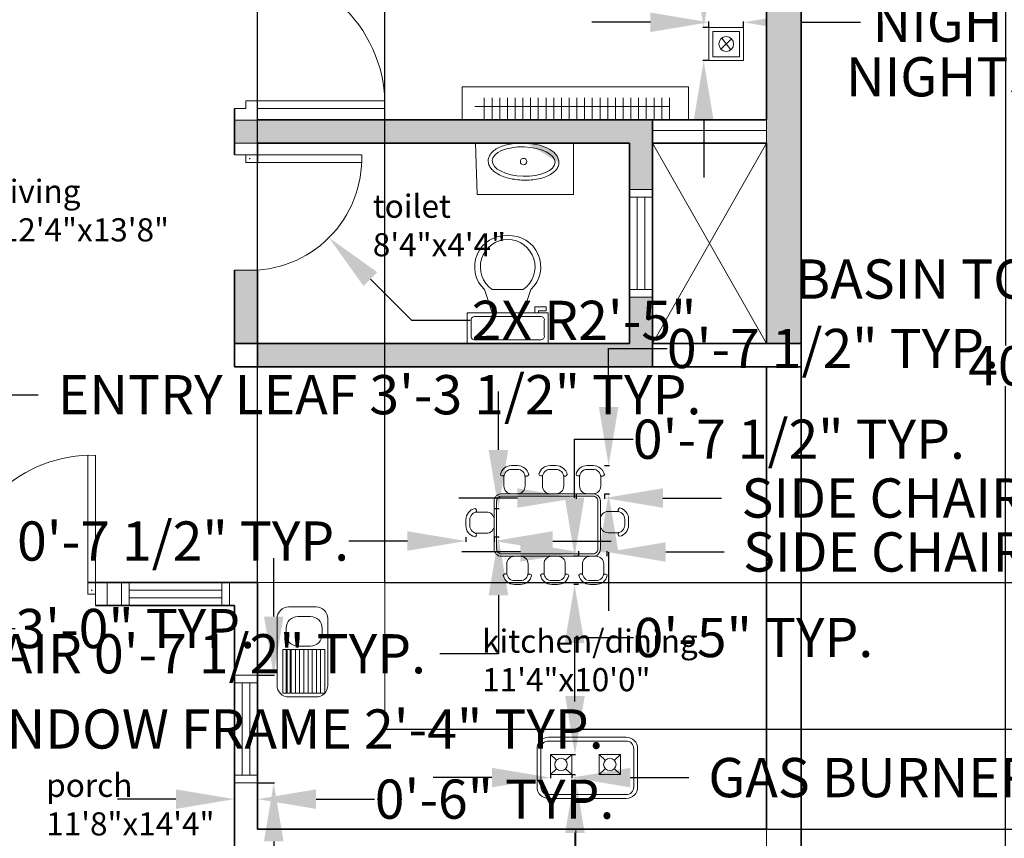
# Model space of a CAD drawing. Units: inches. Extents: x 19 to 15718, y 7 to 930.
# Tile 4 of 11: x 14988 to 15243, y 468 to 680. Entities that reach past the tile are written whole.
import ezdxf

# ---------------------------------------------------------------- set-up
doc = ezdxf.new("R2010")
doc.units = ezdxf.units.IN
doc.header["$MEASUREMENT"] = 0
for name, color, linetype, lineweight in [('A-ANNO-DIMS', 2, 'Continuous', 18), ('A-AREA-IDEN', 7, 'Continuous', 18), ('A-DOOR', 4, 'Continuous', 20), ('A-EQPM', 9, 'Continuous', 18), ('A-FLOR-CASE', 8, 'Continuous', 18), ('A-FLOR-FIXT', 9, 'Continuous', 18), ('A-FLOR-OPEN', 8, 'Continuous', 13), ('A-FURN', 8, 'Continuous', 18), ('A-GLAZ', 4, 'Continuous', 18), ('A-WALL', 7, 'Continuous', 35)]:
    doc.layers.add(name, color=color, linetype=linetype, lineweight=lineweight)
doc.layers.add('A-WALL-PATT', color=18, linetype='Continuous', lineweight=13, true_color=0x000000)
doc.styles.add('Annotative', font='arial.ttf')
doc.styles.get("Standard").update_dxf_attribs({"font": 'arial.ttf'})
doc.dimstyles.get("Standard").update_dxf_attribs({"dimtxt": 10.18, "dimasz": 15.18, "dimexe": 0.18, "dimexo": 0.0625, "dimgap": 0.09, "dimtad": 0, "dimtih": 1, "dimtoh": 1, "dimdec": 0, "dimzin": 0, "dimdsep": 46, "dimlunit": 3, "dimtxsty": 'Standard', "dimcen": 0.09, "dimadec": 0, "dimazin": 0, "dimtfac": 1, "dimtdec": 0, "dimtofl": 0, "dimtmove": 0, "dimatfit": 3, "dimfxl": 1, "dimtolj": 1, "dimtzin": 0, "dimarcsym": 0})

# ---------------------------------------------------------------- blocks, each defined once
blk = doc.blocks.new('*U2')
for p, q in [((9.5, -6), (9.5, -2)), ((-10, -8.5), (-8, -8.5)), ((-10, -9.5), (-10, -8.5)), ((-7, -9.5), (-10, -9.5)), ((-8, -8.5), (-8, -8)), ((-7, -8), (-7, -9.5)), ((-4, -8), (-6, -14)), ((4, -8), (6, -14)), ((4, -14), (-4, -14))]:
    blk.add_line(p, q)
blk.add_lwpolyline([(10.5, -8), (10.5, 0), (-10.5, 0), (-10.5, -8)], close=True)
for points in [[(-9.5, -2), (-9.5, -6)], [(8.5, -1), (-8.5, -1)], [(-8.5, -7), (8.5, -7)]]:
    blk.add_lwpolyline(points)
for centre, radius, start, end in [((-8.625, -1.875), 0.8839, 81.8699, 188.1301), ((8.625, -1.875), 0.8839, 351.8699, 98.1301), ((-8.625, -6.125), 0.8839, 171.869898, 278.1301), ((8.625, -6.125), 0.8839, 261.8699, 8.1301), ((-0.4772, -19.9188), 8.0953, 133.01722, 273.38), ((0.0374, -19.8731), 7.127, 124.50543, 269.7), ((-0.0373, -19.8731), 7.127, 270.3, 55.4946), ((0.4773, -19.9188), 8.0953, 266.62, 46.9828)]:
    blk.add_arc(centre, radius, start, end)
blk = doc.blocks.new('*D17')
at = {"layer": 'A-ANNO-DIMS', "color": 0, "lineweight": -2, "transparency": 16777216}
for p, q in [((15266.62, 830.27), (15243.58, 830.27)), ((15243.76, 815.09), (15243.76, 595.52)), ((15243.76, 365.38), (15243.76, 584.95)), ((15266.62, 350.2), (15243.58, 350.2))]:
    blk.add_line(p, q, dxfattribs=at)
at = {"layer": 'A-ANNO-DIMS', "color": 0, "transparency": 16777216}
for points in [[(15241.23, 815.09), (15246.29, 815.09), (15243.76, 830.27)], [(15241.23, 365.38), (15246.29, 365.38), (15243.76, 350.2)]]:
    blk.add_solid(points, dxfattribs=at)
at = {"layer": 'Defpoints', "color": 0, "transparency": 16777216}
for p in [(15266.68, 830.27), (15243.76, 350.2), (15266.68, 350.2)]:
    blk.add_point(p, dxfattribs=at)
at = {"layer": 'A-ANNO-DIMS', "color": 0, "transparency": 16777216, "insert": (15243.76, 590.24), "char_height": 10.18, "attachment_point": 5}
blk.add_mtext("\\A1;40'", dxfattribs=at)
blk = doc.blocks.new('DOOR-SWING-36IN')
for p, q in [((34.01, 3), (34.01, 39)), ((36.01, 6), (36.01, 39)), ((0.01, 6), (0.01, 0)), ((34.01, 6), (39.01, 6)), ((39.01, 6), (39.01, 0)), ((34.01, 3), (36.01, 3)), ((36.01, 3), (36.01, 0))]:
    blk.add_line(p, q)
blk.add_arc((35.01, 4), 35.01, 88.3634, 181.6366)
blk = doc.blocks.new('WIN-24IN-FRAME6')
for p, q in [((0, 28), (6, 28)), ((0, 26), (6, 26)), ((2, 26), (2, 2)), ((4, 26), (4, 2)), ((0, 2), (6, 2)), ((0, 0), (6, 0))]:
    blk.add_line(p, q)
blk = doc.blocks.new('CHAIR-DINING-LONG-SIDE-A')
blk.add_lwpolyline([(0, 5.06, -0.34468), (2.91, 7.33), (4.42, 7.33, -0.353049), (7.35, 4.97, -0.353049)], format="xyb")
blk.add_lwpolyline([(0.91, 4.33, -0.414214), (2.91, 6.33), (4.42, 6.33, -0.414214), (6.42, 4.33), (6.42, 2, -0.414214), (4.42, 0), (2.91, 0, -0.414214), (0.91, 2)], format="xyb", close=True)
for centre, radius, start, end in [((0.54, 5.15), 0.548, 190.2724, 321.8719), ((6.8, 5.16), 0.588, 223.9333, 340.5026)]:
    blk.add_arc(centre, radius, start, end)
blk = doc.blocks.new('CHAIR-DINING-LONG-SIDE-B')
blk.add_lwpolyline([(6.44, 3, -0.414214), (4.44, 1), (2.93, 1, -0.414214), (0.93, 3), (0.93, 5.33, -0.414214), (2.93, 7.33), (4.44, 7.33, -0.414214), (6.44, 5.33)], format="xyb", close=True)
blk.add_lwpolyline([(7.35, 2.28, -0.34468), (4.44, 0), (2.93, 0, -0.353049), (0, 2.37, -0.353049)], format="xyb")
for centre, radius, start, end in [((0.55, 2.17), 0.588, 43.9333, 160.5026), ((6.81, 2.18), 0.548, 10.2724, 141.8719)]:
    blk.add_arc(centre, radius, start, end)
blk = doc.blocks.new('CHAIR-DINING-END')
blk.add_lwpolyline([(4.33, 6.44, -0.414214), (6.33, 4.44), (6.33, 2.93, -0.414214), (4.33, 0.93), (2, 0.93, -0.414214), (0, 2.93), (0, 4.44, -0.414214), (2, 6.44)], format="xyb", close=True)
blk.add_lwpolyline([(5.06, 7.35, -0.34468), (7.33, 4.44), (7.33, 2.93, -0.353049), (4.97, 0, -0.353049)], format="xyb")
for centre, radius, start, end in [((5.15, 6.81), 0.548, 100.2724, 231.8719), ((5.16, 0.55), 0.588, 133.9333, 250.5026)]:
    blk.add_arc(centre, radius, start, end)
blk = doc.blocks.new('NIGHTSTAND-SQUARE')
for p, q in [((5.89, 5.61), (3.09, 2.97)), ((3.32, 5.82), (5.66, 2.76)), ((3.09, 2.97), (3.09, 2.97))]:
    blk.add_line(p, q)
for points in [[(0, 8.58), (8.98, 8.58), (8.98, 0), (0, 0)], [(1, 7.58), (7.98, 7.58), (7.98, 1), (1, 1)]]:
    blk.add_lwpolyline(points, close=True)
blk.add_circle((4.49, 4.29), 1.92)
blk = doc.blocks.new('HOB-GAS-BURNER')
for p, q in [((0, 5.15), (1.58, 3.68)), ((3.94, 3.69), (5.54, 5.15)), ((1.58, 3.68), (1.58, 3.68)), ((0, 0), (1.58, 1.47)), ((5.54, 0), (3.95, 1.47))]:
    blk.add_line(p, q)
blk.add_lwpolyline([(0, 5.15), (0, 5.15), (5.54, 5.15), (5.54, 5.15), (5.54, 0), (5.54, 0), (0, 0), (0, 0)], close=True)
blk.add_circle((2.77, 2.57), 1.62)
blk = doc.blocks.new('*D36')
at = {"layer": 'A-ANNO-DIMS', "color": 0, "lineweight": -2, "transparency": 16777216}
for p, q in [((15054.04, 525.18), (15054.04, 540.36)), ((15049.9, 510), (15054.22, 510)), ((15049.9, 482), (15054.22, 482)), ((15054.04, 466.82), (15054.04, 451.64))]:
    blk.add_line(p, q, dxfattribs=at)
at = {"layer": 'A-ANNO-DIMS', "color": 0, "transparency": 16777216}
for points in [[(15051.51, 525.18), (15056.57, 525.18), (15054.04, 510)], [(15051.51, 466.82), (15056.57, 466.82), (15054.04, 482)]]:
    blk.add_solid(points, dxfattribs=at)
at = {"layer": 'Defpoints', "color": 0, "transparency": 16777216}
for p in [(15049.84, 510), (15054.04, 510), (15049.84, 482)]:
    blk.add_point(p, dxfattribs=at)
at = {"layer": 'A-ANNO-DIMS', "color": 0, "transparency": 16777216, "insert": (15054.04, 496), "char_height": 10.18, "attachment_point": 5}
blk.add_mtext('\\A1;WINDOW FRAME 2\'-4" TYP.', dxfattribs=at)
blk = doc.blocks.new('*D37')
at = {"layer": 'A-ANNO-DIMS', "color": 0, "lineweight": -2, "transparency": 16777216}
for p, q in [((15043.84, 481.93), (15043.84, 477.62)), ((15049.84, 481.93), (15049.84, 477.62)), ((15028.66, 477.8), (15013.48, 477.8)), ((15065.02, 477.8), (15080.2, 477.8))]:
    blk.add_line(p, q, dxfattribs=at)
at = {"layer": 'A-ANNO-DIMS', "color": 0, "transparency": 16777216}
for points in [[(15028.66, 480.33), (15028.66, 475.27), (15043.84, 477.8)], [(15065.02, 480.33), (15065.02, 475.27), (15049.84, 477.8)]]:
    blk.add_solid(points, dxfattribs=at)
at = {"layer": 'Defpoints', "color": 0, "transparency": 16777216}
for p in [(15043.84, 482), (15049.84, 482), (15049.84, 477.8)]:
    blk.add_point(p, dxfattribs=at)
at = {"layer": 'A-ANNO-DIMS', "color": 0, "transparency": 16777216, "insert": (15111.31, 477.8), "char_height": 10.18, "attachment_point": 5}
blk.add_mtext('\\A1;0\'-6" TYP.', dxfattribs=at)
blk = doc.blocks.new('*D40')
at = {"layer": 'A-ANNO-DIMS', "color": 0, "lineweight": -2, "transparency": 16777216}
for p, q in [((15132.43, 556.96), (15132.43, 555.74)), ((15139.78, 556.96), (15139.78, 555.74)), ((15117.25, 555.92), (15102.07, 555.92)), ((15154.96, 555.92), (15170.14, 555.92))]:
    blk.add_line(p, q, dxfattribs=at)
at = {"layer": 'A-ANNO-DIMS', "color": 0, "transparency": 16777216}
for points in [[(15117.25, 558.45), (15117.25, 553.39), (15132.43, 555.92)], [(15154.96, 558.45), (15154.96, 553.39), (15139.78, 555.92)]]:
    blk.add_solid(points, dxfattribs=at)
at = {"layer": 'Defpoints', "color": 0, "transparency": 16777216}
for p in [(15132.43, 557.02), (15139.78, 557.02), (15139.78, 555.92)]:
    blk.add_point(p, dxfattribs=at)
at = {"layer": 'A-ANNO-DIMS', "color": 0, "transparency": 16777216, "insert": (15262.49, 555.92), "char_height": 10.18, "attachment_point": 5}
blk.add_mtext('\\A1;SIDE CHAIR A 0\'-7 1/2" TYP.', dxfattribs=at)
blk = doc.blocks.new('*D41')
at = {"layer": 'A-ANNO-DIMS', "color": 0, "lineweight": -2, "transparency": 16777216}
for p, q in [((15140.89, 579.54), (15140.89, 594.72)), ((15140.89, 594.72), (15156.07, 594.72)), ((15139.85, 564.36), (15141.07, 564.36)), ((15139.85, 557.02), (15141.07, 557.02)), ((15140.89, 541.84), (15140.89, 526.66))]:
    blk.add_line(p, q, dxfattribs=at)
at = {"layer": 'A-ANNO-DIMS', "color": 0, "transparency": 16777216}
for points in [[(15138.36, 579.54), (15143.42, 579.54), (15140.89, 564.36)], [(15138.36, 541.84), (15143.42, 541.84), (15140.89, 557.02)]]:
    blk.add_solid(points, dxfattribs=at)
at = {"layer": 'Defpoints', "color": 0, "transparency": 16777216}
for p in [(15139.78, 564.36), (15140.89, 564.36), (15139.78, 557.02)]:
    blk.add_point(p, dxfattribs=at)
at = {"layer": 'A-ANNO-DIMS', "color": 0, "transparency": 16777216, "insert": (15199.04, 594.72), "char_height": 10.18, "attachment_point": 5}
blk.add_mtext('\\A1;0\'-7 1/2" TYP.', dxfattribs=at)
blk = doc.blocks.new('*D42')
at = {"layer": 'A-ANNO-DIMS', "color": 0, "lineweight": -2, "transparency": 16777216}
for p, q in [((15117.99, 541.92), (15102.81, 541.92)), ((15133.17, 540.88), (15133.17, 542.1)), ((15140.52, 540.88), (15140.52, 542.1)), ((15155.7, 541.92), (15170.88, 541.92))]:
    blk.add_line(p, q, dxfattribs=at)
at = {"layer": 'A-ANNO-DIMS', "color": 0, "transparency": 16777216}
for points in [[(15117.99, 544.45), (15117.99, 539.39), (15133.17, 541.92)], [(15155.7, 544.45), (15155.7, 539.39), (15140.52, 541.92)]]:
    blk.add_solid(points, dxfattribs=at)
at = {"layer": 'Defpoints', "color": 0, "transparency": 16777216}
for p in [(15140.52, 541.92), (15133.17, 540.82), (15140.52, 540.82)]:
    blk.add_point(p, dxfattribs=at)
at = {"layer": 'A-ANNO-DIMS', "color": 0, "transparency": 16777216, "insert": (15263.22, 541.92), "char_height": 10.18, "attachment_point": 5}
blk.add_mtext('\\A1;SIDE CHAIR B 0\'-7 1/2" TYP.', dxfattribs=at)
blk = doc.blocks.new('*D43')
at = {"layer": 'A-ANNO-DIMS', "color": 0, "lineweight": -2, "transparency": 16777216}
for p, q in [((15132.06, 556), (15132.06, 571.18)), ((15132.06, 571.18), (15147.24, 571.18)), ((15133.1, 540.82), (15131.88, 540.82)), ((15133.1, 533.49), (15131.88, 533.49)), ((15132.06, 518.31), (15132.06, 503.13))]:
    blk.add_line(p, q, dxfattribs=at)
at = {"layer": 'A-ANNO-DIMS', "color": 0, "transparency": 16777216}
for points in [[(15129.53, 556), (15134.59, 556), (15132.06, 540.82)], [(15129.53, 518.31), (15134.59, 518.31), (15132.06, 533.49)]]:
    blk.add_solid(points, dxfattribs=at)
at = {"layer": 'Defpoints', "color": 0, "transparency": 16777216}
for p in [(15132.06, 540.82), (15133.17, 540.82), (15133.17, 533.49)]:
    blk.add_point(p, dxfattribs=at)
at = {"layer": 'A-ANNO-DIMS', "color": 0, "transparency": 16777216, "insert": (15190.22, 571.18), "char_height": 10.18, "attachment_point": 5}
blk.add_mtext('\\A1;0\'-7 1/2" TYP.', dxfattribs=at)
blk = doc.blocks.new('*D46')
at = {"layer": 'A-ANNO-DIMS', "color": 0, "lineweight": -2, "transparency": 16777216}
for p, q in [((15358.25, 608.29), (15358.25, 612.91)), ((15388.25, 608.29), (15388.25, 612.91)), ((15343.07, 612.73), (15327.89, 612.73)), ((15403.43, 612.73), (15418.61, 612.73))]:
    blk.add_line(p, q, dxfattribs=at)
at = {"layer": 'A-ANNO-DIMS', "color": 0, "transparency": 16777216}
for points in [[(15343.07, 615.26), (15343.07, 610.2), (15358.25, 612.73)], [(15403.43, 615.26), (15403.43, 610.2), (15388.25, 612.73)]]:
    blk.add_solid(points, dxfattribs=at)
at = {"layer": 'Defpoints', "color": 0, "transparency": 16777216}
for p in [(15358.25, 612.73), (15358.25, 608.23), (15388.25, 608.23)]:
    blk.add_point(p, dxfattribs=at)
at = {"layer": 'A-ANNO-DIMS', "color": 0, "transparency": 16777216, "insert": (15257.09, 612.73), "char_height": 10.18, "attachment_point": 5}
blk.add_mtext('\\A1;BASIN TOP 2\'-6" TYP.', dxfattribs=at)
blk = doc.blocks.new('*D50')
at = {"layer": 'A-ANNO-DIMS', "color": 0, "lineweight": -2, "transparency": 16777216}
for p, q in [((14977.77, 567.55), (14977.77, 582.73)), ((14977.77, 582.73), (14992.95, 582.73)), ((14971.9, 567.55), (14977.95, 567.55)), ((14977.77, 543.18), (14977.77, 552.37)), ((14971.9, 528), (14977.95, 528))]:
    blk.add_line(p, q, dxfattribs=at)
at = {"layer": 'A-ANNO-DIMS', "color": 0, "transparency": 16777216}
for points in [[(14975.24, 552.37), (14980.3, 552.37), (14977.77, 567.55)], [(14975.24, 543.18), (14980.3, 543.18), (14977.77, 528)]]:
    blk.add_solid(points, dxfattribs=at)
at = {"layer": 'Defpoints', "color": 0, "transparency": 16777216}
for p in [(14971.84, 567.55), (14977.77, 567.55), (14971.84, 528)]:
    blk.add_point(p, dxfattribs=at)
at = {"layer": 'A-ANNO-DIMS', "color": 0, "transparency": 16777216, "insert": (15081.49, 582.73), "char_height": 10.18, "attachment_point": 5}
blk.add_mtext('\\A1;ENTRY LEAF 3\'-3 1/2" TYP.', dxfattribs=at)
blk = doc.blocks.new('*D51')
at = {"layer": 'A-ANNO-DIMS', "color": 0, "lineweight": -2, "transparency": 16777216}
for p, q in [((14935.84, 527.93), (14935.84, 521.88)), ((14971.84, 527.93), (14971.84, 521.88)), ((14951.02, 522.06), (14956.66, 522.06)), ((14971.84, 522.06), (14987.02, 522.06))]:
    blk.add_line(p, q, dxfattribs=at)
at = {"layer": 'A-ANNO-DIMS', "color": 0, "transparency": 16777216}
for points in [[(14951.02, 524.59), (14951.02, 519.53), (14935.84, 522.06)], [(14956.66, 524.59), (14956.66, 519.53), (14971.84, 522.06)]]:
    blk.add_solid(points, dxfattribs=at)
at = {"layer": 'Defpoints', "color": 0, "transparency": 16777216}
for p in [(14935.84, 528), (14971.84, 528), (14971.84, 522.06)]:
    blk.add_point(p, dxfattribs=at)
at = {"layer": 'A-ANNO-DIMS', "color": 0, "transparency": 16777216, "insert": (15018.13, 522.06), "char_height": 10.18, "attachment_point": 5}
blk.add_mtext('\\A1;3\'-0" TYP.', dxfattribs=at)
blk = doc.blocks.new('*D54')
at = {"layer": 'A-ANNO-DIMS', "color": 0, "lineweight": -2, "transparency": 16777216}
for p, q in [((15112.3, 568.4), (15112.3, 583.58)), ((15111.26, 553.22), (15112.48, 553.22)), ((15111.26, 545.87), (15112.48, 545.87)), ((15112.3, 530.69), (15112.3, 515.51)), ((15112.3, 515.51), (15097.12, 515.51))]:
    blk.add_line(p, q, dxfattribs=at)
at = {"layer": 'A-ANNO-DIMS', "color": 0, "transparency": 16777216}
for points in [[(15109.77, 568.4), (15114.83, 568.4), (15112.3, 553.22)], [(15109.77, 530.69), (15114.83, 530.69), (15112.3, 545.87)]]:
    blk.add_solid(points, dxfattribs=at)
at = {"layer": 'Defpoints', "color": 0, "transparency": 16777216}
for p in [(15111.2, 553.22), (15111.2, 545.87), (15112.3, 545.87)]:
    blk.add_point(p, dxfattribs=at)
at = {"layer": 'A-ANNO-DIMS', "color": 0, "transparency": 16777216, "insert": (15013.32, 515.51), "char_height": 10.18, "attachment_point": 5}
blk.add_mtext('\\A1;END CHAIR 0\'-7 1/2" TYP.', dxfattribs=at)
blk = doc.blocks.new('*D55')
at = {"layer": 'A-ANNO-DIMS', "color": 0, "lineweight": -2, "transparency": 16777216}
for p, q in [((15088.69, 544.76), (15073.51, 544.76)), ((15103.87, 545.8), (15103.87, 544.58)), ((15111.2, 545.8), (15111.2, 544.58)), ((15126.38, 544.76), (15141.56, 544.76))]:
    blk.add_line(p, q, dxfattribs=at)
at = {"layer": 'A-ANNO-DIMS', "color": 0, "transparency": 16777216}
for points in [[(15088.69, 547.29), (15088.69, 542.23), (15103.87, 544.76)], [(15126.38, 547.29), (15126.38, 542.23), (15111.2, 544.76)]]:
    blk.add_solid(points, dxfattribs=at)
at = {"layer": 'Defpoints', "color": 0, "transparency": 16777216}
for p in [(15103.87, 545.87), (15103.87, 544.76), (15111.2, 545.87)]:
    blk.add_point(p, dxfattribs=at)
at = {"layer": 'A-ANNO-DIMS', "color": 0, "transparency": 16777216, "insert": (15030.53, 544.76), "char_height": 10.18, "attachment_point": 5}
blk.add_mtext('\\A1;0\'-7 1/2" TYP.', dxfattribs=at)
blk = doc.blocks.new('*D56')
at = {"layer": 'A-ANNO-DIMS', "color": 0, "lineweight": -2, "transparency": 16777216}
for p, q in [((15151.7, 679.35), (15136.52, 679.35)), ((15166.88, 678.06), (15166.88, 679.53)), ((15175.86, 678.06), (15175.86, 679.53)), ((15191.04, 679.35), (15206.22, 679.35))]:
    blk.add_line(p, q, dxfattribs=at)
at = {"layer": 'A-ANNO-DIMS', "color": 0, "transparency": 16777216}
for points in [[(15151.7, 681.88), (15151.7, 676.82), (15166.88, 679.35)], [(15191.04, 681.88), (15191.04, 676.82), (15175.86, 679.35)]]:
    blk.add_solid(points, dxfattribs=at)
at = {"layer": 'Defpoints', "color": 0, "transparency": 16777216}
for p in [(15175.86, 679.35), (15166.88, 678), (15175.86, 678)]:
    blk.add_point(p, dxfattribs=at)
at = {"layer": 'A-ANNO-DIMS', "color": 0, "transparency": 16777216, "insert": (15285.29, 679.35), "char_height": 10.18, "attachment_point": 5}
blk.add_mtext('\\A1;NIGHTSTAND 0\'-9" TYP.', dxfattribs=at)
blk = doc.blocks.new('*D57')
at = {"layer": 'A-ANNO-DIMS', "color": 0, "lineweight": -2, "transparency": 16777216}
for p, q in [((15165.53, 693.18), (15165.53, 708.36)), ((15165.53, 708.36), (15180.71, 708.36)), ((15166.82, 678), (15165.35, 678)), ((15166.82, 669.42), (15165.35, 669.42)), ((15165.53, 654.24), (15165.53, 639.06))]:
    blk.add_line(p, q, dxfattribs=at)
at = {"layer": 'A-ANNO-DIMS', "color": 0, "transparency": 16777216}
for points in [[(15163, 693.18), (15168.06, 693.18), (15165.53, 678)], [(15163, 654.24), (15168.06, 654.24), (15165.53, 669.42)]]:
    blk.add_solid(points, dxfattribs=at)
at = {"layer": 'Defpoints', "color": 0, "transparency": 16777216}
for p in [(15165.53, 678), (15166.88, 678), (15166.88, 669.42)]:
    blk.add_point(p, dxfattribs=at)
at = {"layer": 'A-ANNO-DIMS', "color": 0, "transparency": 16777216, "insert": (15223.69, 708.36), "char_height": 10.18, "attachment_point": 5}
blk.add_mtext('\\A1;0\'-8 1/2" TYP.', dxfattribs=at)
blk = doc.blocks.new('*D58')
at = {"layer": 'A-ANNO-DIMS', "color": 0, "lineweight": -2, "transparency": 16777216}
for p, q in [((15278.41, 688.79), (15278.41, 703.97)), ((15280.87, 673.61), (15278.23, 673.61)), ((15280.87, 656.82), (15278.23, 656.82)), ((15278.41, 641.64), (15278.41, 626.46))]:
    blk.add_line(p, q, dxfattribs=at)
at = {"layer": 'A-ANNO-DIMS', "color": 0, "transparency": 16777216}
for points in [[(15275.88, 688.79), (15280.94, 688.79), (15278.41, 673.61)], [(15275.88, 641.64), (15280.94, 641.64), (15278.41, 656.82)]]:
    blk.add_solid(points, dxfattribs=at)
at = {"layer": 'Defpoints', "color": 0, "transparency": 16777216}
for p in [(15278.41, 673.61), (15280.93, 673.61), (15280.93, 656.82)]:
    blk.add_point(p, dxfattribs=at)
at = {"layer": 'A-ANNO-DIMS', "color": 0, "transparency": 16777216, "insert": (15278.41, 665.21), "char_height": 10.18, "attachment_point": 5}
blk.add_mtext('\\A1;NIGHTSTAND 1\'-5" TYP.', dxfattribs=at)
blk = doc.blocks.new('*D60')
at = {"layer": 'A-ANNO-DIMS', "color": 0, "lineweight": -2, "transparency": 16777216}
for p, q in [((15110.6, 483.39), (15095.42, 483.39)), ((15125.78, 484.16), (15125.78, 483.21)), ((15131.32, 484.16), (15131.32, 483.21)), ((15146.5, 483.39), (15161.68, 483.39))]:
    blk.add_line(p, q, dxfattribs=at)
at = {"layer": 'A-ANNO-DIMS', "color": 0, "transparency": 16777216}
for points in [[(15110.6, 485.92), (15110.6, 480.86), (15125.78, 483.39)], [(15146.5, 485.92), (15146.5, 480.86), (15131.32, 483.39)]]:
    blk.add_solid(points, dxfattribs=at)
at = {"layer": 'Defpoints', "color": 0, "transparency": 16777216}
for p in [(15125.78, 484.23), (15131.32, 484.23), (15131.32, 483.39)]:
    blk.add_point(p, dxfattribs=at)
at = {"layer": 'A-ANNO-DIMS', "color": 0, "transparency": 16777216, "insert": (15253.56, 483.39), "char_height": 10.18, "attachment_point": 5}
blk.add_mtext('\\A1;GAS BURNER 0\'-5 1/2" TYP.', dxfattribs=at)
blk = doc.blocks.new('*D61')
at = {"layer": 'A-ANNO-DIMS', "color": 0, "lineweight": -2, "transparency": 16777216}
for p, q in [((15132.15, 504.55), (15132.15, 519.73)), ((15132.15, 519.73), (15147.33, 519.73)), ((15131.38, 489.37), (15132.33, 489.37)), ((15131.38, 484.23), (15132.33, 484.23)), ((15132.15, 469.05), (15132.15, 453.87))]:
    blk.add_line(p, q, dxfattribs=at)
at = {"layer": 'A-ANNO-DIMS', "color": 0, "transparency": 16777216}
for points in [[(15129.62, 504.55), (15134.68, 504.55), (15132.15, 489.37)], [(15129.62, 469.05), (15134.68, 469.05), (15132.15, 484.23)]]:
    blk.add_solid(points, dxfattribs=at)
at = {"layer": 'Defpoints', "color": 0, "transparency": 16777216}
for p in [(15131.32, 489.37), (15132.15, 489.37), (15131.32, 484.23)]:
    blk.add_point(p, dxfattribs=at)
at = {"layer": 'A-ANNO-DIMS', "color": 0, "transparency": 16777216, "insert": (15178.44, 519.73), "char_height": 10.18, "attachment_point": 5}
blk.add_mtext('\\A1;0\'-5" TYP.', dxfattribs=at)
blk = doc.blocks.new('*D78')
at = {"layer": 'A-ANNO-DIMS', "color": 0, "lineweight": -2, "transparency": 16777216}
for p, q in [((15049.84, 534.06), (15049.84, 923.53)), ((15065.02, 923.35), (15067.65, 923.35)), ((15082.83, 534.06), (15082.83, 923.53)), ((15082.83, 923.35), (15098.01, 923.35))]:
    blk.add_line(p, q, dxfattribs=at)
at = {"layer": 'A-ANNO-DIMS', "color": 0, "transparency": 16777216}
for points in [[(15065.02, 925.88), (15065.02, 920.82), (15049.84, 923.35)], [(15067.65, 925.88), (15067.65, 920.82), (15082.83, 923.35)]]:
    blk.add_solid(points, dxfattribs=at)
at = {"layer": 'Defpoints', "color": 0, "transparency": 16777216}
for p in [(15082.83, 923.35), (15049.84, 534), (15082.83, 534)]:
    blk.add_point(p, dxfattribs=at)
at = {"layer": 'A-ANNO-DIMS', "color": 0, "transparency": 16777216, "insert": (15111.72, 923.35), "char_height": 10.18, "attachment_point": 5}
blk.add_mtext('\\A1;2\'-9"', dxfattribs=at)
blk = doc.blocks.new('*D79')
at = {"layer": 'A-ANNO-DIMS', "color": 0, "lineweight": -2, "transparency": 16777216}
for p, q in [((15602.03, 534), (15602.03, 549.18)), ((15602.03, 549.18), (15617.21, 549.18)), ((15082.89, 534), (15602.21, 534)), ((15602.03, 511.14), (15602.03, 518.82)), ((15082.89, 495.96), (15602.21, 495.96))]:
    blk.add_line(p, q, dxfattribs=at)
at = {"layer": 'A-ANNO-DIMS', "color": 0, "transparency": 16777216}
for points in [[(15599.5, 518.82), (15604.56, 518.82), (15602.03, 534)], [(15599.5, 511.14), (15604.56, 511.14), (15602.03, 495.96)]]:
    blk.add_solid(points, dxfattribs=at)
at = {"layer": 'Defpoints', "color": 0, "transparency": 16777216}
for p in [(15082.83, 534), (15602.03, 534), (15082.83, 495.96)]:
    blk.add_point(p, dxfattribs=at)
at = {"layer": 'A-ANNO-DIMS', "color": 0, "transparency": 16777216, "insert": (15630.83, 549.18), "char_height": 10.18, "attachment_point": 5}
blk.add_mtext('\\A1;3\'-2"', dxfattribs=at)
blk = doc.blocks.new('*D80')
at = {"layer": 'A-ANNO-DIMS', "color": 0, "lineweight": -2, "transparency": 16777216}
for p, q in [((15602.030581, 511.142303), (15602.030581, 526.322303)), ((15181.899116, 495.962303), (15602.210581, 495.962303)), ((15181.899116, 469.995573), (15602.210581, 469.995573)), ((15602.030581, 454.815573), (15602.030581, 439.635573))]:
    blk.add_line(p, q, dxfattribs=at)
at = {"layer": 'A-ANNO-DIMS', "color": 0, "transparency": 16777216}
for points in [[(15599.500581, 511.142303), (15604.560581, 511.142303), (15602.030581, 495.962303)], [(15599.500581, 454.815573), (15604.560581, 454.815573), (15602.030581, 469.995573)]]:
    blk.add_solid(points, dxfattribs=at)
at = {"layer": 'Defpoints', "color": 0, "transparency": 16777216}
for p in [(15181.836616, 495.962303), (15602.030581, 495.962303), (15181.836616, 469.995573)]:
    blk.add_point(p, dxfattribs=at)
at = {"layer": 'A-ANNO-DIMS', "color": 0, "transparency": 16777216, "insert": (15602.030581, 482.978938), "char_height": 10.18, "attachment_point": 5}
blk.add_mtext('\\A1;2\'-2"', dxfattribs=at)
blk = doc.blocks.new('*D87')
at = {"layer": 'A-ANNO-DIMS', "color": 0, "lineweight": -2, "transparency": 16777216}
for p, q in [((14946.77, 579.52), (14961.95, 579.52)), ((14961.95, 579.52), (14972.37, 568.49)), ((15006.75, 532), (15006.93, 532)), ((15006.84, 531.91), (15006.84, 532.09))]:
    blk.add_line(p, q, dxfattribs=at)
at = {"layer": 'A-ANNO-DIMS', "color": 0, "transparency": 16777216}
blk.add_solid([(14974.21, 570.22), (14970.53, 566.75), (14982.79, 557.45)], dxfattribs=at)
at = {"layer": 'Defpoints', "color": 0, "transparency": 16777216}
for p in [(14982.79, 557.45), (15006.84, 532)]:
    blk.add_point(p, dxfattribs=at)
at = {"layer": 'A-ANNO-DIMS', "color": 0, "transparency": 16777216, "insert": (14913.39, 579.52), "char_height": 10.18, "attachment_point": 5}
blk.add_mtext('\\A1;5X R2\'-11"', dxfattribs=at)
blk = doc.blocks.new('*D88')
at = {"layer": 'A-ANNO-DIMS', "color": 0, "lineweight": -2, "transparency": 16777216}
for p, q in [((15047.75, 644), (15047.93, 644)), ((15047.84, 643.91), (15047.84, 644.09)), ((15089.82, 602.01), (15079.09, 612.74)), ((15105, 602.01), (15089.82, 602.01))]:
    blk.add_line(p, q, dxfattribs=at)
at = {"layer": 'A-ANNO-DIMS', "color": 0, "transparency": 16777216}
blk.add_solid([(15080.88, 614.53), (15077.3, 610.95), (15068.35, 623.48)], dxfattribs=at)
at = {"layer": 'Defpoints', "color": 0, "transparency": 16777216}
for p in [(15047.84, 644), (15068.35, 623.48)]:
    blk.add_point(p, dxfattribs=at)
at = {"layer": 'A-ANNO-DIMS', "color": 0, "transparency": 16777216, "insert": (15134.52, 602.01), "char_height": 10.18, "attachment_point": 5}
blk.add_mtext('\\A1;2X R2\'-5"', dxfattribs=at)

msp = doc.modelspace()

# ---------------------------------------------------------------- hatches: boundary and pattern name
at = {"layer": 'A-WALL-PATT'}
h = msp.add_hatch(color=256, dxfattribs=at)
h.dxf.hatch_style = 1
h.paths.add_polyline_path([(15190.84, 837), (14890.84, 837), (14890.84, 357), (14899.84, 357), (14899.84, 366), (14899.84, 528), (14904.84, 528), (14904.84, 534), (14899.84, 534), (14899.84, 698), (15004.84, 698), (15004.84, 701, -0.014283), (15004.84, 703), (15004.84, 704), (14899.84, 704), (14899.84, 828), (14987.26, 828), (15043.84, 828), (15049.84, 828), (15075.84, 828), (15081.84, 828), (15181.84, 828), (15181.84, 780), (15114.84, 780), (15114.84, 779, -0.017236), (15114.84, 777), (15114.84, 774), (15181.84, 774), (15181.84, 654), (15181.84, 648), (15181.84, 596), (15190.84, 596)])
h.paths.add_polyline_path([(15190.84, 590), (15181.84, 590), (15181.84, 470), (15181.84, 464), (15181.84, 361.43), (14991.9, 361.43), (14991.5, 357), (15190.84, 357)], flags=0)
h.paths.add_polyline_path([(15152.29, 608), (15146.29, 608), (15146.29, 596), (15049.84, 596), (15049.84, 590), (15152.29, 590)], flags=17)
h.paths.add_polyline_path([(15049.84, 615), (15048.84, 615, -0.017236), (15046.84, 615), (15043.84, 615), (15043.84, 596), (15049.84, 596)], flags=17)
edge = h.paths.add_edge_path(flags=17)
edge.add_line((15152.29, 654), (15049.84, 654))
edge.add_line((15049.84, 654), (15043.84, 654))
edge.add_line((15043.84, 654), (15043.84, 648))
edge.add_line((15043.84, 648), (15049.84, 648))
edge.add_line((15049.84, 648), (15075.84, 648))
edge.add_line((15075.84, 648), (15081.84, 648))
edge.add_line((15081.84, 648), (15117.26, 648))
edge.add_spline(control_points=[(15117.26, 648), (15117.59, 648.02), (15117.94, 648.03), (15118.71, 648.04), (15119.15, 648.02), (15119.59, 648)], knot_values=[1.499122, 1.499122, 1.499122, 1.499122, 1.618335, 1.618335, 1.770388, 1.770388, 1.770388, 1.770388], degree=3, periodic=0)
edge.add_spline(control_points=[(15127.99, 642.93), (15128, 643.28), (15127.95, 643.62), (15127.73, 644.26), (15127.57, 644.57), (15127.16, 645.13), (15126.92, 645.39), (15126.04, 646.16), (15125.28, 646.6), (15123.53, 647.31), (15122.55, 647.59), (15120.88, 647.88), (15120.24, 647.95), (15119.59, 648)], knot_values=[0, 0, 0, 0, 0.172075, 0.172075, 0.344149, 0.344149, 0.516224, 0.516224, 0.894541, 0.894541, 1.272858, 1.272858, 1.499122, 1.499122, 1.499122, 1.499122], degree=3, periodic=0)
edge.add_line((15119.59, 648), (15146.29, 648))
edge.add_line((15146.29, 648), (15146.29, 636))
edge.add_line((15146.29, 636), (15152.29, 636))
edge.add_line((15152.29, 636), (15152.29, 654))
h.paths.add_polyline_path([(15132.35, 430.4), (15123.35, 430.4), (15123.35, 396.8), (15027.77, 396.8), (15027.77, 387.8), (15132.35, 387.8)], flags=17)
h.paths.add_polyline_path([(15132.35, 464), (15123.35, 464), (15123.35, 430.4), (15132.35, 430.4)], flags=17)
h.paths.add_polyline_path([(15275.68, 583.59), (15276.07, 583.2), (15276.65, 583.2), (15280.6, 587.16), (15278.55, 589.2), (15275.68, 589.2), (15275.68, 601.2), (15266.68, 601.2), (15266.68, 350.2), (15275.68, 350.2), (15275.68, 359.2), (15275.68, 457.2), (15413.68, 457.2), (15413.68, 471.04), (15407.68, 471.04), (15407.68, 463.2), (15275.68, 463.2)])

# ---------------------------------------------------------------- linework, layer by layer
at = {"layer": 'A-DOOR'}
for p, q in [((15049.84, 648), (15043.84, 648)), ((15049.84, 645), (15043.84, 645)), ((15046.84, 645), (15076.84, 645)), ((15046.84, 643), (15046.84, 645)), ((15046.84, 643), (15076.84, 643)), ((15049.84, 615), (15043.84, 615)), ((15005.84, 531), (15005.84, 567)), ((15007.84, 531), (15007.84, 567)), ((15007.84, 534), (15007.84, 528)), ((15010.84, 534), (15010.84, 528)), ((15007.84, 531), (15005.84, 531))]:
    msp.add_line(p, q, dxfattribs=at)
for centre, radius, start, end in [((15047.84, 644), 29.02, 268.0251, 1.9749), ((15006.84, 532), 35.01, 88.3634, 178.3634)]:
    msp.add_arc(centre, radius, start, end, dxfattribs=at)
at = {"layer": 'A-EQPM'}
for points in [[(15148.41, 490.88, 0.414214), (15145.41, 493.88), (15125.31, 493.88, 0.414214), (15122.31, 490.88), (15122.31, 480.96, 0.414214), (15125.31, 477.96), (15145.41, 477.96, 0.414214), (15148.41, 480.96)], [(15147.41, 490.88, 0.414214), (15145.41, 492.88), (15125.31, 492.88, 0.414214), (15123.31, 490.88), (15123.31, 480.96, 0.414214), (15125.31, 478.96), (15145.41, 478.96, 0.414214), (15147.41, 480.96)]]:
    msp.add_lwpolyline(points, format="xyb", close=True, dxfattribs=at)
at = {"layer": 'A-FLOR-CASE'}
for p, q in [((15108.65, 659.73), (15108.65, 654)), ((15110.65, 659.73), (15110.65, 654)), ((15112.65, 659.73), (15112.65, 654)), ((15114.65, 659.73), (15114.65, 654)), ((15116.65, 659.73), (15116.65, 654)), ((15118.65, 659.73), (15118.65, 654)), ((15120.65, 659.73), (15120.65, 654)), ((15122.65, 659.73), (15122.65, 654)), ((15124.65, 659.73), (15124.65, 654)), ((15126.65, 659.73), (15126.65, 654)), ((15128.65, 659.73), (15128.65, 654)), ((15130.65, 659.73), (15130.65, 654)), ((15132.65, 659.73), (15132.65, 654)), ((15134.65, 659.73), (15134.65, 654)), ((15136.65, 659.73), (15136.65, 654)), ((15138.65, 659.73), (15138.65, 654)), ((15140.65, 659.73), (15140.65, 654)), ((15142.65, 659.73), (15142.65, 654)), ((15144.65, 659.73), (15144.65, 654)), ((15146.65, 659.73), (15146.65, 654)), ((15148.65, 659.73), (15148.65, 654)), ((15150.65, 659.73), (15150.65, 654)), ((15152.65, 659.73), (15152.65, 654)), ((15154.65, 659.73), (15154.65, 654)), ((15156.65, 659.73), (15156.65, 654)), ((15106.23, 657.53), (15156.54, 657.53)), ((15049.84, 534), (15082.83, 534)), ((15082.83, 534), (15082.83, 495.96)), ((15082.83, 495.96), (15181.84, 495.96))]:
    msp.add_line(p, q, dxfattribs=at)
msp.add_lwpolyline([(15102.93, 654), (15161.63, 654), (15161.63, 662.6), (15102.93, 662.6)], close=True, dxfattribs=at)
at = {"layer": 'A-FLOR-FIXT'}
for p, q in [((15106.4, 648), (15106.81, 634.63)), ((15131.79, 634.63), (15131.79, 648)), ((15106.81, 634.63), (15131.79, 634.63))]:
    msp.add_line(p, q, dxfattribs=at)
for points in [[(15054.91, 524.65, -0.414214), (15057.91, 527.65), (15065.06, 527.65, -0.414214), (15068.06, 524.65), (15068.06, 507.31, -0.414214), (15065.06, 504.31), (15057.91, 504.31, -0.414214), (15054.91, 507.31)], [(15057.27, 522.19, -0.414214), (15060.27, 525.19), (15063.58, 525.19, -0.414214), (15066.58, 522.19), (15066.58, 520.51, -0.414214), (15063.58, 517.51), (15060.27, 517.51, -0.414214), (15057.27, 520.51)]]:
    msp.add_lwpolyline(points, format="xyb", close=True, dxfattribs=at)
for points in [[(15056.41, 516.58), (15056.41, 516.58), (15057.5, 516.58), (15057.5, 516.58), (15057.5, 505.33), (15057.5, 505.33), (15056.41, 505.33), (15056.41, 505.33)], [(15057.23, 516.58), (15057.23, 516.58), (15058.32, 516.58), (15058.32, 516.58), (15058.32, 505.33), (15058.32, 505.33), (15057.23, 505.33), (15057.23, 505.33)], [(15058.59, 516.58), (15058.59, 516.58), (15059.67, 516.58), (15059.67, 516.58), (15059.67, 505.33), (15059.67, 505.33), (15058.59, 505.33), (15058.59, 505.33)], [(15059.67, 516.58), (15059.67, 516.58), (15060.76, 516.58), (15060.76, 516.58), (15060.76, 505.33), (15060.76, 505.33), (15059.67, 505.33), (15059.67, 505.33)], [(15060.76, 516.58), (15060.76, 516.58), (15061.85, 516.58), (15061.85, 516.58), (15061.85, 505.33), (15061.85, 505.33), (15060.76, 505.33), (15060.76, 505.33)], [(15061.85, 516.58), (15061.85, 516.58), (15062.93, 516.58), (15062.93, 516.58), (15062.93, 505.33), (15062.93, 505.33), (15061.85, 505.33), (15061.85, 505.33)], [(15062.93, 516.58), (15062.93, 516.58), (15064.02, 516.58), (15064.02, 516.58), (15064.02, 505.33), (15064.02, 505.33), (15062.93, 505.33), (15062.93, 505.33)], [(15064.02, 516.58), (15064.02, 516.58), (15065.11, 516.58), (15065.11, 516.58), (15065.11, 505.33), (15065.11, 505.33), (15064.02, 505.33), (15064.02, 505.33)], [(15065.11, 516.58), (15065.11, 516.58), (15066.2, 516.58), (15066.2, 516.58), (15066.2, 505.33), (15066.2, 505.33), (15065.11, 505.33), (15065.11, 505.33)], [(15066.2, 516.58), (15066.2, 516.58), (15067.28, 516.58), (15067.28, 516.58), (15067.28, 505.33), (15067.28, 505.33), (15066.2, 505.33), (15066.2, 505.33)]]:
    msp.add_lwpolyline(points, close=True, dxfattribs=at)
msp.add_circle((15118.83, 643.21), 0.832, dxfattribs=at)
msp.add_ellipse((15118.83, 643.21), major_axis=(8.16, -0.24), ratio=0.467476, dxfattribs=at)
msp.add_open_spline([(15127.99, 642.93), (15128, 643.28), (15127.95, 643.62), (15127.73, 644.26), (15127.57, 644.57), (15127.16, 645.13), (15126.92, 645.39), (15126.04, 646.16), (15125.28, 646.6), (15123.53, 647.31), (15122.55, 647.59), (15120.46, 647.95), (15119.36, 648.04), (15116.95, 648.02), (15115.65, 647.87), (15113.3, 647.28), (15112.26, 646.86), (15111.01, 646), (15110.65, 645.67), (15110.06, 644.92), (15109.84, 644.49), (15109.65, 643.67), (15109.64, 643.28), (15109.77, 642.54), (15109.91, 642.18), (15110.3, 641.53), (15110.54, 641.23), (15111.12, 640.68), (15111.44, 640.43), (15112.68, 639.64), (15113.77, 639.2), (15116.17, 638.59), (15117.49, 638.42), (15120.14, 638.36), (15121.46, 638.47), (15123.87, 638.97), (15124.95, 639.36), (15126.33, 640.18), (15126.77, 640.51), (15127.41, 641.22), (15127.64, 641.58), (15127.91, 642.28), (15127.98, 642.6), (15127.99, 642.93)], degree=3, knots=[0, 0, 0, 0, 0.172075, 0.172075, 0.344149, 0.344149, 0.516224, 0.516224, 0.894541, 0.894541, 1.272858, 1.272858, 1.651176, 1.651176, 2.112724, 2.112724, 2.574273, 2.574273, 2.811208, 2.811208, 3.048143, 3.048143, 3.238272, 3.238272, 3.428401, 3.428401, 3.61853, 3.61853, 3.808659, 3.808659, 4.268108, 4.268108, 4.727558, 4.727558, 5.187007, 5.187007, 5.646456, 5.646456, 5.906091, 5.906091, 6.116999, 6.116999, 6.283185, 6.283185, 6.283185, 6.283185], dxfattribs=at)
at = {"layer": 'A-FLOR-OPEN'}
for p, q in [((15152.29, 648), (15181.84, 596)), ((15181.84, 648), (15152.29, 596))]:
    msp.add_line(p, q, dxfattribs=at)
at = {"layer": 'A-FURN'}
for points in [[(15111.2, 555.13, -0.414214), (15113.09, 557.02), (15136.85, 557.02, -0.414214), (15138.75, 555.13), (15138.75, 542.72, -0.414214), (15136.85, 540.82), (15113.09, 540.82, -0.414214), (15111.2, 542.72)], [(15111.83, 555.13, -0.414214), (15113.09, 556.39), (15136.85, 556.39, -0.414214), (15138.12, 555.13), (15138.12, 542.72, -0.414214), (15136.85, 541.45), (15113.09, 541.45, -0.414214), (15111.83, 542.72)]]:
    msp.add_lwpolyline(points, format="xyb", close=True, dxfattribs=at)
at = {"layer": 'A-GLAZ'}
for p, q in [((15181.84, 654), (15181.84, 648)), ((15152.29, 651.25), (15181.84, 651.25)), ((15132.35, 464), (15132.35, 470)), ((15181.84, 470), (15181.84, 464))]:
    msp.add_line(p, q, dxfattribs=at)
at = {"layer": 'A-WALL'}
for p, q in [((15190.84, 837), (15190.84, 357)), ((15181.84, 774), (15181.84, 654)), ((15043.84, 645), (15043.84, 657)), ((15049.84, 654), (15181.84, 654)), ((15152.29, 654), (15152.29, 590)), ((15049.84, 648), (15075.84, 648)), ((15049.84, 643), (15049.84, 648)), ((15075.84, 648), (15081.84, 648)), ((15081.84, 648), (15146.29, 648)), ((15146.29, 648), (15146.29, 596)), ((15152.29, 648), (15181.84, 648)), ((15181.84, 648), (15181.84, 596)), ((15043.84, 590), (15043.84, 615)), ((15049.84, 590), (15049.84, 615.05)), ((15043.84, 596), (15146.29, 596)), ((15152.29, 596), (15190.84, 596)), ((15043.84, 590), (15190.84, 590)), ((15181.84, 590), (15181.84, 470)), ((15005.84, 534), (15043.84, 534)), ((15043.84, 534), (15043.84, 534)), ((15043.84, 534), (15049.84, 534)), ((15049.84, 470), (15049.84, 534)), ((15049.84, 534), (15049.84, 534)), ((15007.84, 528), (15043.84, 528)), ((15043.84, 464), (15043.84, 528)), ((15049.84, 470), (15181.84, 470))]:
    msp.add_line(p, q, dxfattribs=at)

# ---------------------------------------------------------------- block references
at = {"layer": 'A-DOOR', "rotation": 269.9999999999929}
msp.add_blockref('DOOR-SWING-36IN', (15043.84, 693), dxfattribs=at)
at = {"layer": 'A-EQPM'}
for p in [(15125.78, 484.22), (15138.43, 484.22)]:
    msp.add_blockref('HOB-GAS-BURNER', p, dxfattribs=at)
at = {"layer": 'A-FLOR-FIXT', "rotation": 180}
msp.add_blockref('*U2', (15114.71, 596), dxfattribs=at)
at = {"layer": 'A-FURN'}
for name, p in [('NIGHTSTAND-SQUARE', (15166.88, 669.42)), ('CHAIR-DINING-LONG-SIDE-A', (15112.81, 557.02)), ('CHAIR-DINING-LONG-SIDE-A', (15122.81, 557.02)), ('CHAIR-DINING-LONG-SIDE-A', (15132.43, 557.02)), ('CHAIR-DINING-END', (15138.75, 545.99)), ('CHAIR-DINING-LONG-SIDE-B', (15113.56, 533.49)), ('CHAIR-DINING-LONG-SIDE-B', (15123.21, 533.49)), ('CHAIR-DINING-LONG-SIDE-B', (15133.17, 533.49))]:
    msp.add_blockref(name, p, dxfattribs=at)
at = {"layer": 'A-FURN', "rotation": 180}
msp.add_blockref('CHAIR-DINING-END', (15111.2, 553.22), dxfattribs=at)
at = {"layer": 'A-GLAZ'}
for p, rotation in [((15152.29, 636), 180), ((15042.55, 528), 90.0000000000073)]:
    msp.add_blockref('WIN-24IN-FRAME6', p, dxfattribs=dict(at, rotation=rotation))
msp.add_blockref('WIN-24IN-FRAME6', (15043.84, 482), dxfattribs=at)

# ---------------------------------------------------------------- texts
at = {"layer": 'A-AREA-IDEN', "char_height": 6, "width": 68.1983, "attachment_point": 1, "style": 'Annotative'}
for s, insert in [('living\\P12\'4"x13\'8"', (14983.24, 638.5)), ('toilet\\P8\'4"x4\'4"', (15079.73, 634.63)), ('kitchen/dining\\P11\'4"x10\'0"', (15108.09, 521.79)), ('porch\\P11\'8"x14\'4"', (14995.03, 484.38))]:
    msp.add_mtext(s, dxfattribs=dict(at, insert=insert))

# ---------------------------------------------------------------- dimensions: what is measured, and where the dimension line sits
at = {"layer": 'A-ANNO-DIMS'}
dim = msp.add_linear_dim(base=(15082.83, 923.35), p1=(15049.84, 534), p2=(15082.83, 534), dimstyle='Standard', override={"dimdec": 1, "dimlfac": 1, "dimrnd": 0, "dimzin": 1, "dimdsep": 46, "dimlunit": 4, "dimfrac": 2}, dxfattribs=at)
dim.commit()
dim.dimension.update_dxf_attribs({"geometry": '*D78', "text_midpoint": (15111.72, 923.35)})
for base, p1, p2, override, picture, middle in [((15243.76, 350.2), (15266.68, 830.27), (15266.68, 350.2), {"dimclrd": 0, "dimclre": 0, "dimclrt": 0}, '*D17', (15243.76, 590.24)), ((15602.03, 534), (15082.83, 495.96), (15082.83, 534), {"dimdec": 1, "dimlfac": 1, "dimrnd": 0, "dimzin": 1, "dimdsep": 46, "dimlunit": 4, "dimfrac": 2}, '*D79', (15630.83, 549.18)), ((15602.03, 495.96), (15181.84, 470), (15181.84, 495.96), {"dimdec": 1, "dimlfac": 1, "dimrnd": 0, "dimzin": 1, "dimdsep": 46, "dimlunit": 4, "dimfrac": 2}, '*D80', (15602.03, 482.98))]:
    dim = msp.add_linear_dim(base=base, p1=p1, p2=p2, angle=90, dimstyle='Standard', override=override, dxfattribs=at)
    dim.commit()
    dim.dimension.update_dxf_attribs({"geometry": picture, "text_midpoint": middle})
for base, p1, p2, angle, text, picture, middle in [((15165.53, 678), (15166.88, 669.42), (15166.88, 678), 90, '<> TYP.', '*D57', (15223.69, 708.36)), ((15278.41, 673.61), (15280.93, 656.82), (15280.93, 673.61), 90, 'NIGHTSTAND <> TYP.', '*D58', (15278.41, 665.21)), ((15358.25, 612.73), (15388.25, 608.23), (15358.25, 608.23), 180, 'BASIN TOP <> TYP.', '*D46', (15257.09, 612.73)), ((14977.7695, 567.5479), (14971.8366, 527.9956), (14971.8366, 567.5479), 90, 'ENTRY LEAF <> TYP.', '*D50', (15081.493, 582.7279)), ((15140.89, 564.36), (15139.78, 557.02), (15139.78, 564.36), 90, '<> TYP.', '*D41', (15199.04, 594.72)), ((15132.06, 540.82), (15133.17, 533.49), (15133.17, 540.82), 90, '<> TYP.', '*D43', (15190.22, 571.18)), ((15112.3017, 545.8656), (15111.1988, 553.2183), (15111.1988, 545.8656), 270, 'END CHAIR <> TYP.', '*D54', (15013.3244, 515.5056)), ((15103.87, 544.76), (15111.2, 545.87), (15103.87, 545.87), 180, '<> TYP.', '*D55', (15030.53, 544.76)), ((15054.04, 510), (15049.84, 482), (15049.84, 510), 90, 'WINDOW FRAME <> TYP.', '*D36', (15054.04, 496)), ((15132.15, 489.37), (15131.32, 484.22), (15131.32, 489.37), 90, '<> TYP.', '*D61', (15178.44, 519.73))]:
    dim = msp.add_linear_dim(base=base, p1=p1, p2=p2, angle=angle, text=text, dimstyle='Standard', override={"dimdec": 1, "dimlfac": 1, "dimrnd": 0, "dimzin": 1, "dimdsep": 46, "dimlunit": 4, "dimfrac": 2}, dxfattribs=at)
    dim.commit()
    dim.dimension.update_dxf_attribs({"geometry": picture, "text_midpoint": middle})
for base, p1, p2, text, picture, middle in [((15175.86, 679.35), (15166.88, 678), (15175.86, 678), 'NIGHTSTAND <> TYP.', '*D56', (15285.29, 679.35)), ((15139.7848, 555.9195), (15132.4322, 557.0224), (15139.7848, 557.0224), 'SIDE CHAIR A <> TYP.', '*D40', (15262.4867, 555.9195)), ((15140.519, 541.924), (15133.1663, 540.8211), (15140.519, 540.8211), 'SIDE CHAIR B <> TYP.', '*D42', (15263.2209, 541.924)), ((14971.84, 522.06), (14935.84, 528), (14971.84, 528), '<> TYP.', '*D51', (15018.13, 522.06)), ((15131.32, 483.39), (15125.78, 484.22), (15131.32, 484.22), 'GAS BURNER <> TYP.', '*D60', (15253.56, 483.39)), ((15049.84, 477.8), (15043.84, 482), (15049.84, 482), '<> TYP.', '*D37', (15111.31, 477.8))]:
    dim = msp.add_linear_dim(base=base, p1=p1, p2=p2, text=text, dimstyle='Standard', override={"dimdec": 1, "dimlfac": 1, "dimrnd": 0, "dimzin": 1, "dimdsep": 46, "dimlunit": 4, "dimfrac": 2}, dxfattribs=at)
    dim.commit()
    dim.dimension.update_dxf_attribs({"geometry": picture, "text_midpoint": middle})
for center, mpoint, text, picture, middle in [((15047.84, 644), (15068.35, 623.48), '2X <>', '*D88', (15134.52, 602.01)), ((15006.84, 532), (14982.79, 557.45), '5X <>', '*D87', (14913.39, 579.52))]:
    dim = msp.add_radius_dim(center=center, mpoint=mpoint, text=text, dimstyle='Standard', override={"dimdec": 1, "dimlfac": 1, "dimrnd": 0, "dimzin": 1, "dimdsep": 46, "dimlunit": 4, "dimfrac": 2}, dxfattribs=at)
    dim.commit()
    dim.dimension.update_dxf_attribs({"geometry": picture, "text_midpoint": middle})

doc.saveas('drawing.dxf')
